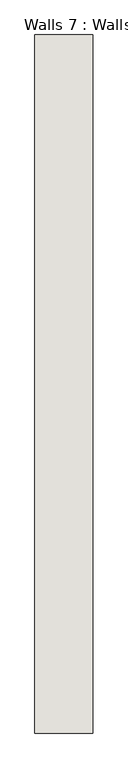
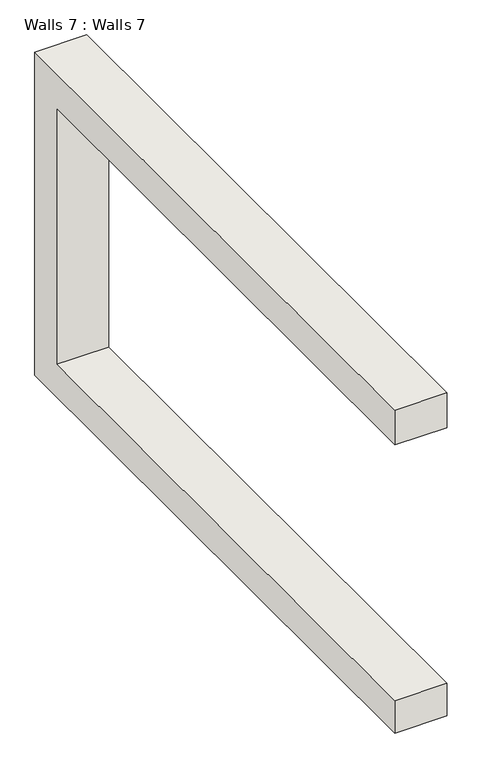
"""IFC4 building model written with IfcOpenShell, lengths in millimetres: wall geometry, Walls 7 : Walls 7."""

from ifc_helpers import new_model, si_unit, frame, origin, place, context, project, spatial, polyline, outline, extrude, source, transform, mapped, element, save


def walls_7_walls_7_556ff675(model_context):
    return source(origin(), model_context, "Body", "SweptSolid", [
        extrude(outline(polyline([(-994.5139512, 6456.6399557), (5829.4327161, 6456.6399557), (5829.4327161, 2723.0941247), (-994.5139512, 2723.0941247), (-994.5139512, 3098.9391777), (5416.1269374, 3098.9391777), (5416.1269374, 6055.6826372), (-994.5139512, 6055.6826372), (-994.5139512, 6456.6399557)])), frame((-9144.8328829, 0.0, 0.0), z_axis=(1.0, 0.0, 0.0), x_axis=(0.0, 1.0, 0.0)), (0.0, 0.0, 1.0), 567.6016928),
    ])


if __name__ == "__main__":
    model = new_model("IFC4")
    model_context = context("Model", 3, world=origin())
    ifc_project = project(units=[si_unit("LENGTHUNIT", "METRE", prefix="MILLI")], contexts=[model_context])
    site = spatial("IfcSite", under=ifc_project)
    building = spatial("IfcBuilding", under=site)
    placement = place(None, origin())
    walls_7_walls_7_shape = walls_7_walls_7_556ff675(model_context)
    element("IfcWall", 1, ObjectType="Walls 7 : Walls 7", at=placement, inside=building, context=model_context, shape_type="MappedRepresentation", body=[
        mapped(walls_7_walls_7_shape, transform((0.0, 0.0, 0.0), x_axis=(1.0, 0.0, 0.0), y_axis=(0.0, 1.0, 0.0), z_axis=(0.0, 0.0, 1.0))),
    ])
    save(model, "model.ifc")

# Revit data of these elements
# Element 1 (IfcWall, "Walls 7 : Walls 7")
#   Materials on its faces: "Default Wall"
# Materials
#   "Default Wall": colour RGB 128 128 128, transparency 0
